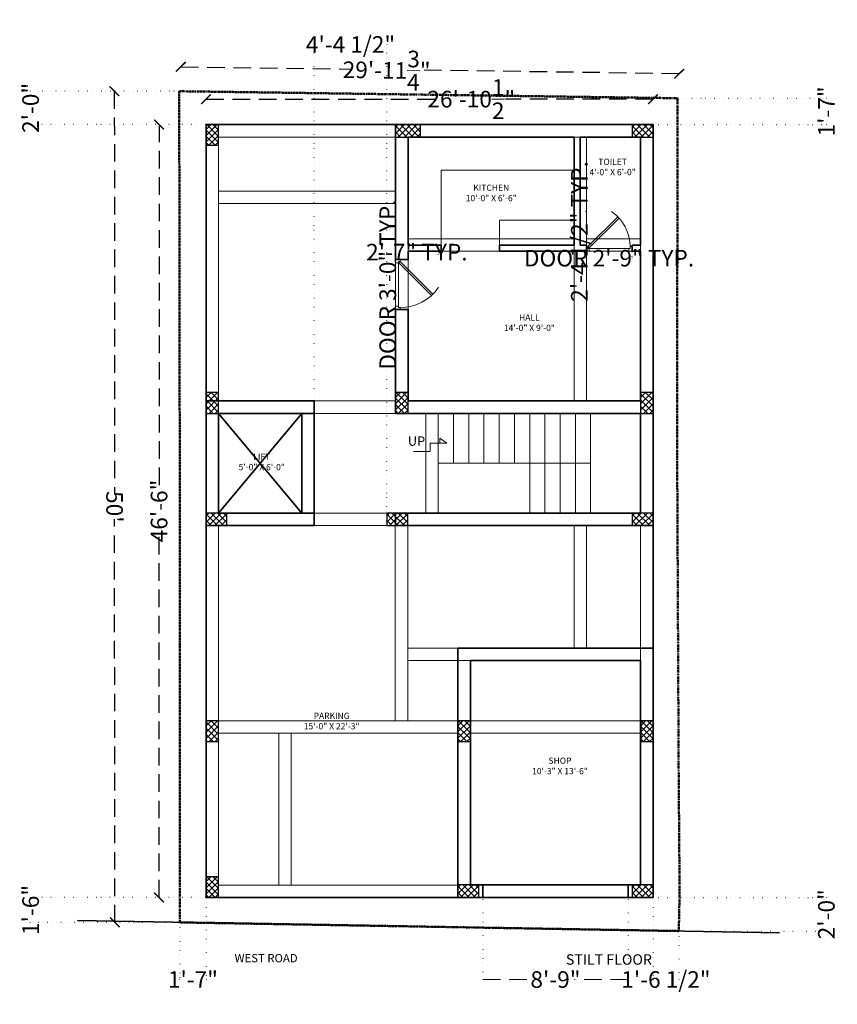
# Model space of a CAD drawing. Units: inches. Extents: x -16911 to -9621, y -48626 to -46270.
# Tile 10 of 20: x -12796 to -12206, y -47022 to -46311. Entities that reach past the tile are written whole.
import ezdxf

# ---------------------------------------------------------------- set-up
doc = ezdxf.new("R2010")
doc.units = ezdxf.units.IN
for name, pattern in [('DASHDOT', [1, 0.5, -0.25, 0, -0.25]), ('DASHED', [19.05, 12.7, -6.35]), ('DOT2', [3.175, 0, -3.175])]:
    doc.linetypes.add(name, pattern=pattern)
for name, color, linetype, lineweight in [('A-ANNO-DIMS', 2, 'Continuous', 13), ('A-ANNO-SYMB', 3, 'Continuous', 13), ('A-ANNO-TEXT', 7, 'Continuous', 18), ('A-AREA-IDEN', 3, 'Continuous', 18), ('A-DOOR', 4, 'Continuous', 18), ('A-FLOR-STRS', 3, 'Continuous', 18), ('A-FURN', 8, 'Continuous', 13), ('A-WALL', 7, 'Continuous', 35), ('C-PROP', 6, 'DASHDOT', 50), ('column', 12, 'Continuous', 30), ('DOOR', 143, 'Continuous', 9), ('EXT BEAM', 132, 'Continuous', 13), ('S-BEAM', 132, 'Continuous', 25), ('S-COLS', 1, 'Continuous', 30), ('STAIRCASE', 137, 'Continuous', 5)]:
    doc.layers.add(name, color=color, linetype=linetype, lineweight=lineweight)
doc.styles.get("Standard").update_dxf_attribs({"font": 'swissel.ttf'})
doc.styles.add('style9', font='swisscl.ttf', dxfattribs={"height": 12})
doc.dimstyles.new('Dim9', dxfattribs={"dimtxt": 10, "dimasz": 0.199219, "dimexe": 1, "dimexo": 0.5, "dimgap": 1, "dimtad": 0, "dimdec": 1, "dimzin": 0, "dimdsep": 46, "dimlunit": 4, "dimtxsty": 'style9', "dimblk": 'ARCHTICK', "dimcen": 0.09, "dimclrd": 256, "dimclrt": 256, "dimadec": 0, "dimazin": 0, "dimtfac": 1, "dimtdec": 1, "dimtix": 1, "dimtofl": 0, "dimtmove": 1, "dimatfit": 3, "dimfxl": 9, "dimtolj": 1, "dimtzin": 0, "dimlwd": -1, "dimarcsym": 0})

# ---------------------------------------------------------------- blocks, each defined once
blk = doc.blocks.new('_ArchTick')
at = {"color": 0, "linetype": 'ByBlock', "const_width": 0.15}
blk.add_lwpolyline([(-0.5, -0.5), (0.5, 0.5)], dxfattribs=at)
blk = doc.blocks.new('*D9')
at = {"layer": 'A-ANNO-DIMS', "color": 0, "linetype": 'DOT2', "lineweight": -2, "transparency": 16777216}
for p, q in [((-12679.71, -46345.34), (-12679.69, -46344.15)), ((-12320.05, -46350.39), (-12320.03, -46349.2))]:
    blk.add_line(p, q, dxfattribs=at)
at = {"layer": 'A-ANNO-DIMS', "color": 0, "linetype": 'DASHED', "lineweight": 25, "transparency": 16777216}
for p, q in [((-12679.71, -46345.15), (-12555.97, -46346.89)), ((-12320.04, -46350.2), (-12506.38, -46347.59))]:
    blk.add_line(p, q, dxfattribs=at)
at = {"layer": 'Defpoints', "color": 0, "transparency": 16777216}
for p in [(-12320.04, -46350.2), (-12679.9, -46359.07), (-12320.24, -46364.11)]:
    blk.add_point(p, dxfattribs=at)
at = {"layer": 'A-ANNO-DIMS', "color": 0, "lineweight": 25, "transparency": 16777216, "xscale": 7, "yscale": 7, "zscale": 7}
for p, rotation in [((-12679.71, -46345.15), 179.1963905603631), ((-12320.04, -46350.2), 359.196390560363)]:
    blk.add_blockref('_ArchTick', p, dxfattribs=dict(at, rotation=rotation))
at = {"layer": 'A-ANNO-DIMS', "color": 0, "transparency": 16777216, "insert": (-12531.18, -46347.68), "char_height": 12, "attachment_point": 5, "rotation": 359.19639, "style": 'style9'}
blk.add_mtext('\\A1;29\'-11{\\H1x;\\S3/4;}"', dxfattribs=at)
blk = doc.blocks.new('*D10')
at = {"layer": 'A-ANNO-DIMS', "color": 0, "linetype": 'DOT2', "lineweight": -2, "transparency": 16777216}
for p, q in [((-12727.5, -46362.82), (-12728.69, -46362.82)), ((-12727.14, -46962.82), (-12728.32, -46962.82))]:
    blk.add_line(p, q, dxfattribs=at)
at = {"layer": 'A-ANNO-DIMS', "color": 0, "linetype": 'DASHED', "lineweight": 25, "transparency": 16777216}
for p, q in [((-12727.69, -46362.82), (-12727.51, -46653.98)), ((-12727.32, -46962.82), (-12727.5, -46671.67))]:
    blk.add_line(p, q, dxfattribs=at)
at = {"layer": 'Defpoints', "color": 0, "transparency": 16777216}
for p in [(-12727.69, -46362.82), (-12708.87, -46362.81), (-12708.51, -46962.81)]:
    blk.add_point(p, dxfattribs=at)
at = {"layer": 'A-ANNO-DIMS', "color": 0, "lineweight": 25, "transparency": 16777216, "xscale": 7, "yscale": 7, "zscale": 7}
for p, rotation in [((-12727.69, -46362.82), 90.0346840750536), ((-12727.32, -46962.82), 270.0346840750536)]:
    blk.add_blockref('_ArchTick', p, dxfattribs=dict(at, rotation=rotation))
at = {"layer": 'A-ANNO-DIMS', "color": 0, "transparency": 16777216, "insert": (-12727.51, -46662.82), "char_height": 12, "attachment_point": 5, "rotation": 270.03468, "style": 'style9'}
blk.add_mtext("\\A1;50'", dxfattribs=at)
blk = doc.blocks.new('*D11')
at = {"layer": 'A-ANNO-DIMS', "color": 0, "linetype": 'DOT2', "lineweight": -2, "transparency": 16777216}
for p, q in [((-12661.47, -46368.33), (-12661.47, -46369.52)), ((-12338.92, -46368.33), (-12338.92, -46369.52))]:
    blk.add_line(p, q, dxfattribs=at)
at = {"layer": 'A-ANNO-DIMS', "color": 0, "linetype": 'DASHED', "lineweight": 25, "transparency": 16777216}
for p, q in [((-12661.47, -46368.52), (-12494.69, -46368.52)), ((-12338.92, -46368.52), (-12445.42, -46368.52))]:
    blk.add_line(p, q, dxfattribs=at)
at = {"layer": 'Defpoints', "color": 0, "transparency": 16777216}
for p in [(-12661.47, -46345.28), (-12338.92, -46345.28), (-12338.92, -46368.52)]:
    blk.add_point(p, dxfattribs=at)
at = {"layer": 'A-ANNO-DIMS', "color": 0, "lineweight": 25, "transparency": 16777216, "xscale": 7, "yscale": 7, "zscale": 7, "rotation": 180}
blk.add_blockref('_ArchTick', (-12661.47, -46368.52), dxfattribs=at)
at = {"layer": 'A-ANNO-DIMS', "color": 0, "lineweight": 25, "transparency": 16777216, "xscale": 7, "yscale": 7, "zscale": 7}
blk.add_blockref('_ArchTick', (-12338.92, -46368.52), dxfattribs=at)
at = {"layer": 'A-ANNO-DIMS', "color": 0, "transparency": 16777216, "insert": (-12470.06, -46368.52), "char_height": 12, "attachment_point": 5, "style": 'style9'}
blk.add_mtext('\\A1;26\'-10{\\H1x;\\S1/2;}"', dxfattribs=at)
blk = doc.blocks.new('*D16')
at = {"layer": 'A-ANNO-DIMS', "color": 0, "linetype": 'DOT2', "lineweight": -2, "transparency": 16777216}
for p, q in [((-12695.22, -46386.86), (-12696.4, -46386.86)), ((-12695.22, -46944.81), (-12696.4, -46944.81))]:
    blk.add_line(p, q, dxfattribs=at)
at = {"layer": 'A-ANNO-DIMS', "color": 0, "linetype": 'DASHED', "lineweight": 25, "transparency": 16777216}
for p, q in [((-12695.4, -46386.86), (-12695.4, -46648.2)), ((-12695.4, -46944.81), (-12695.4, -46683.47))]:
    blk.add_line(p, q, dxfattribs=at)
at = {"layer": 'Defpoints', "color": 0, "transparency": 16777216}
for p in [(-12661.47, -46386.86), (-12695.4, -46944.81), (-12661.47, -46944.81)]:
    blk.add_point(p, dxfattribs=at)
at = {"layer": 'A-ANNO-DIMS', "color": 0, "lineweight": 25, "transparency": 16777216, "xscale": 7, "yscale": 7, "zscale": 7}
for p, rotation in [((-12695.4, -46386.86), 90), ((-12695.4, -46944.81), 270)]:
    blk.add_blockref('_ArchTick', p, dxfattribs=dict(at, rotation=rotation))
at = {"layer": 'A-ANNO-DIMS', "color": 0, "transparency": 16777216, "insert": (-12695.4, -46665.83), "char_height": 12, "attachment_point": 5, "rotation": 90, "style": 'style9'}
blk.add_mtext('\\A1;46\'-6"', dxfattribs=at)
blk = doc.blocks.new('THYHYTJ')
at = {"layer": 'STAIRCASE', "ltscale": 10}
for p, q in [((-7981.18, -46346.18), (-7984.62, -46351.1)), ((-7981.18, -46358.18), (-7981.18, -46346.18)), ((-7984.62, -46351.1), (-7981.18, -46351.1)), ((-7975.18, -46358.18), (-7981.18, -46358.18)), ((-7975.18, -46370.18), (-7975.18, -46358.18))]:
    blk.add_line(p, q, dxfattribs=at)
blk = doc.blocks.new('A$C1C9D3E54')
at = {"layer": 'DOOR'}
blk.add_line((18676.53, 5780.72), (18710.53, 5780.72), dxfattribs=at)
blk.add_lwpolyline([(18685.01, 5806.62), (18710.47, 5781.16), (18711.53, 5782.22), (18686.07, 5807.68), (18685.01, 5806.62)], dxfattribs=at)
blk.add_lwpolyline([(18674.03, 5778.22), (18676.03, 5778.22), (18674.03, 5778.22), (18674.03, 5782.22), (18675.53, 5782.22), (18675.53, 5780.72), (18676.53, 5780.72), (18676.53, 5778.72), (18676.41, 5778.72), (18676.41, 5778.6, -0.414214), (18676.16, 5778.35), (18676.03, 5778.35), (18676.03, 5778.22)], format="xyb", dxfattribs=at)
blk.add_lwpolyline([(18713.03, 5782.22), (18711.53, 5782.22), (18711.53, 5780.72), (18710.53, 5780.72), (18710.53, 5778.72), (18710.66, 5778.72), (18710.66, 5778.6, 0.414214), (18710.91, 5778.35), (18711.03, 5778.35), (18711.03, 5778.22), (18713.03, 5778.22), (18711.03, 5778.22), (18713.03, 5778.22), (18713.03, 5782.22)], format="xyb", close=True, dxfattribs=at)
blk.add_arc((18711.53, 5782.22), 36, 124.03362, 180, dxfattribs=at)
blk = doc.blocks.new('COLUMNS')
at = {"layer": 'column'}
h = blk.add_hatch(dxfattribs=at)
h.set_pattern_fill('ANSI37', color=256, angle=-720)
h.set_pattern_definition([(45, (21703.4588, -104481.6704), (-2.24506403, 2.24506403), []), (135, (21703.4588, -104481.6704), (-2.24506403, -2.24506403), [])])
h.paths.add_polyline_path([(-12061.47, -46401.86), (-12052.47, -46401.86), (-12052.47, -46386.86), (-12061.47, -46386.86)])
h = blk.add_hatch(dxfattribs=at)
h.set_pattern_fill('ANSI37', color=256, angle=-810)
h.set_pattern_definition([(315, (-70004.5392, -80151.7886), (2.24506403, 2.24506403), []), (45, (-70004.5392, -80151.7886), (-2.24506403, 2.24506403), [])])
h.paths.add_polyline_path([(-11924.72, -46386.86), (-11924.72, -46395.86), (-11906.72, -46395.86), (-11906.72, -46386.86)])
h = blk.add_hatch(dxfattribs=at)
h.set_pattern_fill('ANSI37', color=256, angle=-810)
h.set_pattern_definition([(315, (-69833.7395, -80151.7886), (2.24506403, 2.24506403), []), (45, (-69833.7395, -80151.7886), (-2.24506403, 2.24506403), [])])
h.paths.add_polyline_path([(-11753.92, -46386.86), (-11753.92, -46395.86), (-11738.92, -46395.86), (-11738.92, -46386.86)])
h = blk.add_hatch(dxfattribs=at)
h.set_pattern_fill('ANSI37', color=256, angle=-900)
h.set_pattern_definition([(225, (-45817.4075, 11499.4594), (2.24506403, -2.24506403), []), (315, (-45817.4075, 11499.4594), (2.24506403, 2.24506403), [])])
h.paths.add_polyline_path([(-12052.47, -46580.36), (-12061.47, -46580.36), (-12061.47, -46595.36), (-12052.47, -46595.36)])
h = blk.add_hatch(dxfattribs=at)
h.set_pattern_fill('ANSI37', color=256, angle=-720)
h.set_pattern_definition([(45, (21840.2088, -104675.1704), (-2.24506403, 2.24506403), []), (135, (21840.2088, -104675.1704), (-2.24506403, -2.24506403), [])])
h.paths.add_polyline_path([(-11924.72, -46595.36), (-11915.72, -46595.36), (-11915.72, -46580.36), (-11924.72, -46580.36)])
h = blk.add_hatch(dxfattribs=at)
h.set_pattern_fill('ANSI37', color=256, angle=-900)
h.set_pattern_definition([(225, (-45503.8578, 11499.4594), (2.24506403, -2.24506403), []), (315, (-45503.8578, 11499.4594), (2.24506403, 2.24506403), [])])
h.paths.add_polyline_path([(-11738.92, -46580.36), (-11747.92, -46580.36), (-11747.92, -46595.36), (-11738.92, -46595.36)])
h = blk.add_hatch(dxfattribs=at)
h.set_pattern_fill('ANSI37', color=256, angle=-810)
h.set_pattern_definition([(315, (-70141.2892, -80432.2886), (2.24506403, 2.24506403), []), (45, (-70141.2892, -80432.2886), (-2.24506403, 2.24506403), [])])
h.paths.add_polyline_path([(-12061.47, -46667.36), (-12061.47, -46676.36), (-12046.47, -46676.36), (-12046.47, -46667.36)])
h = blk.add_hatch(dxfattribs=at)
h.set_pattern_fill('ANSI37', color=256, angle=-810)
h.set_pattern_definition([(315, (-70010.7892, -80432.2886), (2.24506403, 2.24506403), []), (45, (-70010.7892, -80432.2886), (-2.24506403, 2.24506403), [])])
h.paths.add_polyline_path([(-11930.97, -46667.36), (-11930.97, -46676.36), (-11915.97, -46676.36), (-11915.97, -46667.36)])
h = blk.add_hatch(dxfattribs=at)
h.set_pattern_fill('ANSI37', color=256, angle=-810)
h.set_pattern_definition([(315, (-69833.7395, -80432.2886), (2.24506403, 2.24506403), []), (45, (-69833.7395, -80432.2886), (-2.24506403, 2.24506403), [])])
h.paths.add_polyline_path([(-11753.92, -46667.36), (-11753.92, -46676.36), (-11738.92, -46676.36), (-11738.92, -46667.36)])
h = blk.add_hatch(dxfattribs=at)
h.set_pattern_fill('ANSI37', color=256, angle=-540)
h.set_pattern_definition([(225, (-45817.4075, 11262.5055), (2.24506403, -2.24506403), []), (315, (-45817.4075, 11262.5055), (2.24506403, 2.24506403), [])])
h.paths.add_polyline_path([(-12052.47, -46817.31), (-12061.47, -46817.31), (-12061.47, -46832.31), (-12052.47, -46832.31)])
h = blk.add_hatch(dxfattribs=at)
h.set_pattern_fill('ANSI37', color=256, angle=-720)
h.set_pattern_definition([(45, (21885.2088, -104912.1242), (-2.24506403, 2.24506403), []), (135, (21885.2088, -104912.1242), (-2.24506403, -2.24506403), [])])
h.paths.add_polyline_path([(-11879.72, -46832.31), (-11870.72, -46832.31), (-11870.72, -46817.31), (-11879.72, -46817.31)])
h = blk.add_hatch(dxfattribs=at)
h.set_pattern_fill('ANSI37', color=256, angle=-720)
h.set_pattern_definition([(45, (22017.1023, -104912.1242), (-2.24506403, 2.24506403), []), (135, (22017.1023, -104912.1242), (-2.24506403, -2.24506403), [])])
h.paths.add_polyline_path([(-11747.83, -46832.31), (-11738.83, -46832.31), (-11738.83, -46817.31), (-11747.83, -46817.31)])
h = blk.add_hatch(dxfattribs=at)
h.set_pattern_fill('ANSI37', color=256, angle=-720)
h.set_pattern_definition([(45, (21703.4588, -105024.6242), (-2.24506403, 2.24506403), []), (135, (21703.4588, -105024.6242), (-2.24506403, -2.24506403), [])])
h.paths.add_polyline_path([(-12061.47, -46944.81), (-12052.47, -46944.81), (-12052.47, -46929.81), (-12061.47, -46929.81)])
h = blk.add_hatch(dxfattribs=at)
h.set_pattern_fill('ANSI37', color=256, angle=-810)
h.set_pattern_definition([(315, (-69959.5392, -80700.7425), (2.24506403, 2.24506403), []), (45, (-69959.5392, -80700.7425), (-2.24506403, 2.24506403), [])])
h.paths.add_polyline_path([(-11879.72, -46935.81), (-11879.72, -46944.81), (-11864.72, -46944.81), (-11864.72, -46935.81)])
h = blk.add_hatch(dxfattribs=at)
h.set_pattern_fill('ANSI37', color=256, angle=-810)
h.set_pattern_definition([(315, (-69833.7395, -80700.7425), (2.24506403, 2.24506403), []), (45, (-69833.7395, -80700.7425), (-2.24506403, 2.24506403), [])])
h.paths.add_polyline_path([(-11753.92, -46935.81), (-11753.92, -46944.81), (-11738.92, -46944.81), (-11738.92, -46935.81)])
at = {"layer": 'column', "ltscale": 0.05}
for points in [[(-12052.47, -46386.86), (-12061.47, -46386.86), (-12061.47, -46401.86), (-12052.47, -46401.86)], [(-11906.72, -46395.86), (-11906.72, -46386.86), (-11924.72, -46386.86), (-11924.72, -46395.86)], [(-11738.92, -46395.86), (-11738.92, -46386.86), (-11753.92, -46386.86), (-11753.92, -46395.86)], [(-12061.47, -46595.36), (-12052.47, -46595.36), (-12052.47, -46580.36), (-12061.47, -46580.36)], [(-11915.72, -46580.36), (-11924.72, -46580.36), (-11924.72, -46595.36), (-11915.72, -46595.36)], [(-11747.92, -46595.36), (-11738.92, -46595.36), (-11738.92, -46580.36), (-11747.92, -46580.36)], [(-12046.47, -46676.36), (-12046.47, -46667.36), (-12061.47, -46667.36), (-12061.47, -46676.36)], [(-11915.97, -46676.36), (-11915.97, -46667.36), (-11930.97, -46667.36), (-11930.97, -46676.36)], [(-11738.92, -46676.36), (-11738.92, -46667.36), (-11753.92, -46667.36), (-11753.92, -46676.36)], [(-12061.47, -46832.31), (-12052.47, -46832.31), (-12052.47, -46817.31), (-12061.47, -46817.31)], [(-11870.72, -46817.31), (-11879.72, -46817.31), (-11879.72, -46832.31), (-11870.72, -46832.31)], [(-11738.83, -46817.31), (-11747.83, -46817.31), (-11747.83, -46832.31), (-11738.83, -46832.31)], [(-12052.47, -46929.81), (-12061.47, -46929.81), (-12061.47, -46944.81), (-12052.47, -46944.81)], [(-11864.72, -46944.81), (-11864.72, -46935.81), (-11879.72, -46935.81), (-11879.72, -46944.81)], [(-11738.92, -46944.81), (-11738.92, -46935.81), (-11753.92, -46935.81), (-11753.92, -46944.81)]]:
    blk.add_lwpolyline(points, close=True, dxfattribs=at)
blk = doc.blocks.new('TYPICAL BEAMS G-2')
at = {"layer": 'EXT BEAM'}
for p, q in [((-12061.47, -47658.74), (-11738.92, -47658.74)), ((-12061.47, -48216.7), (-12061.47, -47658.74)), ((-11738.92, -48216.7), (-11738.92, -47658.74)), ((-12052.47, -47667.74), (-11924.72, -47667.74)), ((-12052.47, -47939.24), (-12052.47, -47667.74)), ((-11924.72, -47667.74), (-11924.72, -47858.24)), ((-11915.72, -47667.74), (-11747.92, -47667.74)), ((-11915.72, -47667.74), (-11915.72, -47858.24)), ((-11795.92, -47667.74), (-11795.92, -47858.24)), ((-11786.92, -47667.74), (-11786.92, -47858.24)), ((-11747.92, -47858.24), (-11747.92, -47667.74)), ((-12052.47, -47706.74), (-11924.72, -47706.74)), ((-12052.47, -47715.74), (-11924.72, -47715.74)), ((-11915.72, -47741.24), (-11795.92, -47741.24)), ((-11786.92, -47741.24), (-11747.92, -47741.24)), ((-11915.72, -47750.24), (-11795.92, -47750.24)), ((-11786.92, -47750.24), (-11747.92, -47750.24)), ((-12052.47, -47858.24), (-11924.72, -47858.24)), ((-11915.72, -47858.24), (-11747.92, -47858.24)), ((-12052.47, -47867.24), (-11924.72, -47867.24)), ((-11992.47, -47867.24), (-11992.47, -47939.24)), ((-11983.47, -47867.24), (-11983.47, -47939.24)), ((-11915.72, -47867.24), (-11747.92, -47867.24)), ((-11902.92, -47867.24), (-11902.92, -47939.24)), ((-11893.92, -47867.24), (-11893.92, -47939.24)), ((-11747.92, -47939.24), (-11747.92, -47867.24)), ((-12046.47, -47939.24), (-11929.47, -47939.24)), ((-11920.47, -47939.24), (-11738.92, -47939.24)), ((-12052.47, -48089.2), (-12052.47, -47948.24)), ((-12046.47, -47948.24), (-11929.47, -47948.24)), ((-11924.97, -47948.24), (-11924.97, -48089.2)), ((-11920.47, -47948.24), (-11738.92, -47948.24)), ((-11915.97, -47948.24), (-11915.97, -48089.2)), ((-11795.92, -47948.24), (-11795.92, -48036.7)), ((-11786.92, -47948.24), (-11786.92, -48036.7)), ((-11747.92, -48089.2), (-11747.92, -47948.24)), ((-11747.92, -48036.7), (-11915.97, -48036.7)), ((-11747.92, -48045.7), (-11915.97, -48045.7)), ((-12052.47, -48089.2), (-11747.92, -48089.2)), ((-12052.47, -48216.7), (-12052.47, -48098.2)), ((-12052.47, -48098.2), (-11879.72, -48098.2)), ((-12008.97, -48098.2), (-12008.97, -48207.7)), ((-11999.97, -48098.2), (-11999.97, -48207.7)), ((-11879.72, -48098.2), (-11879.72, -48207.7)), ((-11870.72, -48098.2), (-11747.92, -48098.2)), ((-11870.72, -48098.2), (-11870.72, -48207.7)), ((-11747.92, -48207.7), (-11747.92, -48098.2)), ((-12052.47, -48207.7), (-11879.72, -48207.7)), ((-11870.72, -48207.7), (-11747.92, -48207.7)), ((-12061.47, -48216.7), (-11738.92, -48216.7))]:
    blk.add_line(p, q, dxfattribs=at)
blk = doc.blocks.new('*D65')
at = {"layer": 'A-ANNO-DIMS', "color": 0, "linetype": 'DOT2', "lineweight": -2, "transparency": 16777216}
for p, q in [((-12525.47, -46484.36), (-12531.37, -46484.36)), ((-12525.47, -46520.36), (-12531.37, -46520.36))]:
    blk.add_line(p, q, dxfattribs=at)
at = {"layer": 'A-ANNO-DIMS', "linetype": 'DASHED', "transparency": 16777216}
for p, q in [((-12530.37, -46484.36), (-12530.37, -46484.16)), ((-12530.37, -46520.36), (-12530.37, -46520.55))]:
    blk.add_line(p, q, dxfattribs=at)
at = {"layer": 'Defpoints', "color": 0, "transparency": 16777216}
for p in [(-12530.37, -46484.36), (-12524.97, -46484.36), (-12524.97, -46520.36)]:
    blk.add_point(p, dxfattribs=at)
at = {"layer": 'A-ANNO-DIMS', "transparency": 16777216, "xscale": 0.19921875, "yscale": 0.19921875, "zscale": 0.19921875}
for p, rotation in [((-12530.37, -46484.36), 270), ((-12530.37, -46520.36), 90)]:
    blk.add_blockref('_ArchTick', p, dxfattribs=dict(at, rotation=rotation))
at = {"layer": 'A-ANNO-DIMS', "transparency": 16777216, "insert": (-12530.37, -46502.36), "char_height": 12, "attachment_point": 5, "rotation": 90, "style": 'style9'}
blk.add_mtext('\\A1;DOOR 3\'-0" TYP.', dxfattribs=at)
blk = doc.blocks.new('*D66')
at = {"layer": 'A-ANNO-DIMS', "linetype": 'DASHED', "transparency": 16777216}
for p, q in [((-12524.97, -46478.96), (-12525.17, -46478.96)), ((-12493.75, -46478.96), (-12493.55, -46478.96))]:
    blk.add_line(p, q, dxfattribs=at)
at = {"layer": 'A-ANNO-DIMS', "color": 0, "linetype": 'DOT2', "lineweight": -2, "transparency": 16777216}
for p, q in [((-12524.97, -46483.86), (-12524.97, -46477.96)), ((-12493.75, -46483.86), (-12493.75, -46477.96))]:
    blk.add_line(p, q, dxfattribs=at)
at = {"layer": 'Defpoints', "color": 0, "transparency": 16777216}
for p in [(-12524.97, -46484.36), (-12493.75, -46478.96), (-12493.75, -46484.36)]:
    blk.add_point(p, dxfattribs=at)
at = {"layer": 'A-ANNO-DIMS', "transparency": 16777216, "xscale": 0.19921875, "yscale": 0.19921875, "zscale": 0.19921875}
blk.add_blockref('_ArchTick', (-12524.97, -46478.96), dxfattribs=at)
at = {"layer": 'A-ANNO-DIMS', "transparency": 16777216, "xscale": 0.19921875, "yscale": 0.19921875, "zscale": 0.19921875, "rotation": 180}
blk.add_blockref('_ArchTick', (-12493.75, -46478.96), dxfattribs=at)
at = {"layer": 'A-ANNO-DIMS', "transparency": 16777216, "insert": (-12509.36, -46478.96), "char_height": 12, "attachment_point": 5, "style": 'style9'}
blk.add_mtext('\\A1;2\'-7" TYP.', dxfattribs=at)
blk = doc.blocks.new('*D67')
at = {"layer": 'A-ANNO-DIMS', "linetype": 'DASHED', "transparency": 16777216}
for p, q in [((-12387.17, -46483.31), (-12387.37, -46483.31)), ((-12354.17, -46483.31), (-12353.98, -46483.31))]:
    blk.add_line(p, q, dxfattribs=at)
at = {"layer": 'A-ANNO-DIMS', "color": 0, "linetype": 'DOT2', "lineweight": -2, "transparency": 16777216}
for p, q in [((-12387.17, -46478.86), (-12387.17, -46484.31)), ((-12354.17, -46478.86), (-12354.17, -46484.31))]:
    blk.add_line(p, q, dxfattribs=at)
at = {"layer": 'Defpoints', "color": 0, "transparency": 16777216}
for p in [(-12387.17, -46478.36), (-12387.17, -46483.31), (-12354.17, -46478.36)]:
    blk.add_point(p, dxfattribs=at)
at = {"layer": 'A-ANNO-DIMS', "transparency": 16777216, "xscale": 0.19921875, "yscale": 0.19921875, "zscale": 0.19921875}
blk.add_blockref('_ArchTick', (-12387.17, -46483.31), dxfattribs=at)
at = {"layer": 'A-ANNO-DIMS', "transparency": 16777216, "xscale": 0.19921875, "yscale": 0.19921875, "zscale": 0.19921875, "rotation": 180}
blk.add_blockref('_ArchTick', (-12354.17, -46483.31), dxfattribs=at)
at = {"layer": 'A-ANNO-DIMS', "transparency": 16777216, "insert": (-12370.67, -46483.31), "char_height": 12, "attachment_point": 5, "style": 'style9'}
blk.add_mtext('\\A1;DOOR 2\'-9" TYP.', dxfattribs=at)
blk = doc.blocks.new('*D68')
at = {"layer": 'A-ANNO-DIMS', "color": 0, "linetype": 'DOT2', "lineweight": -2, "transparency": 16777216}
for p, q in [((-12387.67, -46449.73), (-12393.12, -46449.73)), ((-12387.67, -46478.36), (-12393.12, -46478.36))]:
    blk.add_line(p, q, dxfattribs=at)
at = {"layer": 'A-ANNO-DIMS', "linetype": 'DASHED', "transparency": 16777216}
for p, q in [((-12392.12, -46449.73), (-12392.12, -46449.53)), ((-12392.12, -46478.36), (-12392.12, -46478.55))]:
    blk.add_line(p, q, dxfattribs=at)
at = {"layer": 'Defpoints', "color": 0, "transparency": 16777216}
for p in [(-12392.12, -46449.73), (-12387.17, -46449.73), (-12387.17, -46478.36)]:
    blk.add_point(p, dxfattribs=at)
at = {"layer": 'A-ANNO-DIMS', "transparency": 16777216, "xscale": 0.19921875, "yscale": 0.19921875, "zscale": 0.19921875}
for p, rotation in [((-12392.12, -46449.73), 270), ((-12392.12, -46478.36), 90)]:
    blk.add_blockref('_ArchTick', p, dxfattribs=dict(at, rotation=rotation))
at = {"layer": 'A-ANNO-DIMS', "transparency": 16777216, "insert": (-12392.12, -46464.04), "char_height": 12, "attachment_point": 5, "rotation": 90, "style": 'style9'}
blk.add_mtext('\\A1;2\'-4 1/2" TYP.', dxfattribs=at)
blk = doc.blocks.new('*D106')
at = {"layer": 'A-ANNO-DIMS', "color": 0, "linetype": 'DOT2', "lineweight": -2, "transparency": 16777216}
for p, q in [((-12681.34, -46362.81), (-12789.1, -46362.81)), ((-12661.97, -46386.86), (-12789.1, -46386.86))]:
    blk.add_line(p, q, dxfattribs=at)
at = {"layer": 'A-ANNO-DIMS', "linetype": 'DASHED', "transparency": 16777216}
for p, q in [((-12788.1, -46362.81), (-12788.1, -46362.61)), ((-12788.1, -46386.86), (-12788.1, -46387.05))]:
    blk.add_line(p, q, dxfattribs=at)
at = {"layer": 'Defpoints', "color": 0, "transparency": 16777216}
for p in [(-12680.84, -46362.81), (-12788.1, -46386.86), (-12661.47, -46386.86)]:
    blk.add_point(p, dxfattribs=at)
at = {"layer": 'A-ANNO-DIMS', "transparency": 16777216, "xscale": 0.19921875, "yscale": 0.19921875, "zscale": 0.19921875}
for p, rotation in [((-12788.1, -46362.81), 270), ((-12788.1, -46386.86), 90)]:
    blk.add_blockref('_ArchTick', p, dxfattribs=dict(at, rotation=rotation))
at = {"layer": 'A-ANNO-DIMS', "transparency": 16777216, "insert": (-12788.1, -46374.83), "char_height": 12, "attachment_point": 5, "rotation": 90, "style": 'style9'}
blk.add_mtext('\\A1;2\'-0"', dxfattribs=at)
blk = doc.blocks.new('*D107')
at = {"layer": 'A-ANNO-DIMS', "color": 0, "linetype": 'DOT2', "lineweight": -2, "transparency": 16777216}
for p, q in [((-12320.67, -46367.86), (-12212.8, -46367.86)), ((-12338.42, -46386.86), (-12212.8, -46386.86))]:
    blk.add_line(p, q, dxfattribs=at)
at = {"layer": 'A-ANNO-DIMS', "linetype": 'DASHED', "transparency": 16777216}
for p, q in [((-12213.8, -46367.86), (-12213.8, -46367.66)), ((-12213.8, -46386.86), (-12213.8, -46387.05))]:
    blk.add_line(p, q, dxfattribs=at)
at = {"layer": 'Defpoints', "color": 0, "transparency": 16777216}
for p in [(-12321.17, -46367.86), (-12338.92, -46386.86), (-12213.8, -46386.86)]:
    blk.add_point(p, dxfattribs=at)
at = {"layer": 'A-ANNO-DIMS', "transparency": 16777216, "xscale": 0.19921875, "yscale": 0.19921875, "zscale": 0.19921875}
for p, rotation in [((-12213.8, -46367.86), 270), ((-12213.8, -46386.86), 90)]:
    blk.add_blockref('_ArchTick', p, dxfattribs=dict(at, rotation=rotation))
at = {"layer": 'A-ANNO-DIMS', "transparency": 16777216, "insert": (-12213.8, -46377.36), "char_height": 12, "attachment_point": 5, "rotation": 90, "style": 'style9'}
blk.add_mtext('\\A1;1\'-7"', dxfattribs=at)
blk = doc.blocks.new('*D108')
at = {"layer": 'A-ANNO-DIMS', "color": 0, "linetype": 'DOT2', "lineweight": -2, "transparency": 16777216}
for p, q in [((-12661.97, -46944.81), (-12789.1, -46944.81)), ((-12680.97, -46962.81), (-12789.1, -46962.81))]:
    blk.add_line(p, q, dxfattribs=at)
at = {"layer": 'A-ANNO-DIMS', "linetype": 'DASHED', "transparency": 16777216}
for p, q in [((-12788.1, -46944.81), (-12788.1, -46944.61)), ((-12788.1, -46962.81), (-12788.1, -46963.01))]:
    blk.add_line(p, q, dxfattribs=at)
at = {"layer": 'Defpoints', "color": 0, "transparency": 16777216}
for p in [(-12788.1, -46944.81), (-12661.47, -46944.81), (-12680.47, -46962.81)]:
    blk.add_point(p, dxfattribs=at)
at = {"layer": 'A-ANNO-DIMS', "transparency": 16777216, "xscale": 0.19921875, "yscale": 0.19921875, "zscale": 0.19921875}
for p, rotation in [((-12788.1, -46944.81), 270), ((-12788.1, -46962.81), 90)]:
    blk.add_blockref('_ArchTick', p, dxfattribs=dict(at, rotation=rotation))
at = {"layer": 'A-ANNO-DIMS', "transparency": 16777216, "insert": (-12788.1, -46953.81), "char_height": 12, "attachment_point": 5, "rotation": 90, "style": 'style9'}
blk.add_mtext('\\A1;1\'-6"', dxfattribs=at)
blk = doc.blocks.new('*D109')
at = {"layer": 'A-ANNO-DIMS', "color": 0, "linetype": 'DOT2', "lineweight": -2, "transparency": 16777216}
for p, q in [((-12338.42, -46944.81), (-12212.8, -46944.81)), ((-12319.79, -46969.03), (-12212.8, -46969.03))]:
    blk.add_line(p, q, dxfattribs=at)
at = {"layer": 'A-ANNO-DIMS', "linetype": 'DASHED', "transparency": 16777216}
for p, q in [((-12213.8, -46944.81), (-12213.8, -46944.61)), ((-12213.8, -46969.03), (-12213.8, -46969.23))]:
    blk.add_line(p, q, dxfattribs=at)
at = {"layer": 'Defpoints', "color": 0, "transparency": 16777216}
for p in [(-12338.92, -46944.81), (-12213.8, -46944.81), (-12320.29, -46969.03)]:
    blk.add_point(p, dxfattribs=at)
at = {"layer": 'A-ANNO-DIMS', "transparency": 16777216, "xscale": 0.19921875, "yscale": 0.19921875, "zscale": 0.19921875}
for p, rotation in [((-12213.8, -46944.81), 270), ((-12213.8, -46969.03), 90)]:
    blk.add_blockref('_ArchTick', p, dxfattribs=dict(at, rotation=rotation))
at = {"layer": 'A-ANNO-DIMS', "transparency": 16777216, "insert": (-12213.8, -46956.92), "char_height": 12, "attachment_point": 5, "rotation": 90, "style": 'style9'}
blk.add_mtext('\\A1;2\'-0"', dxfattribs=at)
blk = doc.blocks.new('*D110')
at = {"layer": 'A-ANNO-DIMS', "color": 0, "linetype": 'DOT2', "lineweight": -2, "transparency": 16777216}
for p, q in [((-12661.47, -46945.31), (-12661.47, -47005.04)), ((-12680.47, -46963.31), (-12680.47, -47005.04))]:
    blk.add_line(p, q, dxfattribs=at)
at = {"layer": 'A-ANNO-DIMS', "linetype": 'DASHED', "transparency": 16777216}
for p, q in [((-12680.47, -47004.04), (-12680.67, -47004.04)), ((-12661.47, -47004.04), (-12661.28, -47004.04))]:
    blk.add_line(p, q, dxfattribs=at)
at = {"layer": 'Defpoints', "color": 0, "transparency": 16777216}
for p in [(-12661.47, -46944.81), (-12680.47, -46962.81), (-12661.47, -47004.04)]:
    blk.add_point(p, dxfattribs=at)
at = {"layer": 'A-ANNO-DIMS', "transparency": 16777216, "xscale": 0.19921875, "yscale": 0.19921875, "zscale": 0.19921875}
blk.add_blockref('_ArchTick', (-12680.47, -47004.04), dxfattribs=at)
at = {"layer": 'A-ANNO-DIMS', "transparency": 16777216, "xscale": 0.19921875, "yscale": 0.19921875, "zscale": 0.19921875, "rotation": 180}
blk.add_blockref('_ArchTick', (-12661.47, -47004.04), dxfattribs=at)
at = {"layer": 'A-ANNO-DIMS', "transparency": 16777216, "insert": (-12670.97, -47004.04), "char_height": 12, "attachment_point": 5, "style": 'style9'}
blk.add_mtext('\\A1;1\'-7"', dxfattribs=at)
blk = doc.blocks.new('*D111')
at = {"layer": 'A-ANNO-DIMS', "color": 0, "linetype": 'DOT2', "lineweight": -2, "transparency": 16777216}
for p, q in [((-12338.92, -46945.31), (-12338.92, -47005.04)), ((-12320.29, -46969.53), (-12320.29, -47005.04))]:
    blk.add_line(p, q, dxfattribs=at)
at = {"layer": 'A-ANNO-DIMS', "linetype": 'DASHED', "transparency": 16777216}
for p, q in [((-12338.92, -47004.04), (-12339.12, -47004.04)), ((-12320.29, -47004.04), (-12320.09, -47004.04))]:
    blk.add_line(p, q, dxfattribs=at)
at = {"layer": 'Defpoints', "color": 0, "transparency": 16777216}
for p in [(-12338.92, -46944.81), (-12320.29, -46969.03), (-12338.92, -47004.04)]:
    blk.add_point(p, dxfattribs=at)
at = {"layer": 'A-ANNO-DIMS', "transparency": 16777216, "xscale": 0.19921875, "yscale": 0.19921875, "zscale": 0.19921875}
blk.add_blockref('_ArchTick', (-12338.92, -47004.04), dxfattribs=at)
at = {"layer": 'A-ANNO-DIMS', "transparency": 16777216, "xscale": 0.19921875, "yscale": 0.19921875, "zscale": 0.19921875, "rotation": 180}
blk.add_blockref('_ArchTick', (-12320.29, -47004.04), dxfattribs=at)
at = {"layer": 'A-ANNO-DIMS', "transparency": 16777216, "insert": (-12329.61, -47004.04), "char_height": 12, "attachment_point": 5, "style": 'style9'}
blk.add_mtext('\\A1;1\'-6 1/2"', dxfattribs=at)
blk = doc.blocks.new('*D112')
at = {"layer": 'A-ANNO-DIMS', "color": 0, "linetype": 'DOT2', "lineweight": -2, "transparency": 16777216}
for p, q in [((-12461.72, -46936.31), (-12461.72, -47005.04)), ((-12356.92, -46936.31), (-12356.92, -47005.04))]:
    blk.add_line(p, q, dxfattribs=at)
at = {"layer": 'A-ANNO-DIMS', "linetype": 'DASHED', "transparency": 16777216}
for p, q in [((-12461.72, -47004.04), (-12423.14, -47004.04)), ((-12356.92, -47004.04), (-12395.51, -47004.04))]:
    blk.add_line(p, q, dxfattribs=at)
at = {"layer": 'Defpoints', "color": 0, "transparency": 16777216}
for p in [(-12461.72, -46935.81), (-12356.92, -46935.81), (-12356.92, -47004.04)]:
    blk.add_point(p, dxfattribs=at)
at = {"layer": 'A-ANNO-DIMS', "transparency": 16777216, "xscale": 0.19921875, "yscale": 0.19921875, "zscale": 0.19921875, "rotation": 180}
blk.add_blockref('_ArchTick', (-12461.72, -47004.04), dxfattribs=at)
at = {"layer": 'A-ANNO-DIMS', "transparency": 16777216, "xscale": 0.19921875, "yscale": 0.19921875, "zscale": 0.19921875}
blk.add_blockref('_ArchTick', (-12356.92, -47004.04), dxfattribs=at)
at = {"layer": 'A-ANNO-DIMS', "transparency": 16777216, "insert": (-12409.32, -47004.04), "char_height": 12, "attachment_point": 5, "style": 'style9'}
blk.add_mtext('\\A1;8\'-9"', dxfattribs=at)
blk = doc.blocks.new('*D113')
at = {"layer": 'A-ANNO-DIMS', "linetype": 'DASHED', "transparency": 16777216}
for p, q in [((-12583.47, -46329.06), (-12583.67, -46329.06)), ((-12530.97, -46329.06), (-12530.78, -46329.06))]:
    blk.add_line(p, q, dxfattribs=at)
at = {"layer": 'A-ANNO-DIMS', "color": 0, "linetype": 'DOT2', "lineweight": -2, "transparency": 16777216}
for p, q in [((-12583.47, -46675.86), (-12583.47, -46328.06)), ((-12530.97, -46675.86), (-12530.97, -46328.06))]:
    blk.add_line(p, q, dxfattribs=at)
at = {"layer": 'Defpoints', "color": 0, "transparency": 16777216}
for p in [(-12530.97, -46329.06), (-12583.47, -46676.36), (-12530.97, -46676.36)]:
    blk.add_point(p, dxfattribs=at)
at = {"layer": 'A-ANNO-DIMS', "transparency": 16777216, "xscale": 0.19921875, "yscale": 0.19921875, "zscale": 0.19921875}
blk.add_blockref('_ArchTick', (-12583.47, -46329.06), dxfattribs=at)
at = {"layer": 'A-ANNO-DIMS', "transparency": 16777216, "xscale": 0.19921875, "yscale": 0.19921875, "zscale": 0.19921875, "rotation": 180}
blk.add_blockref('_ArchTick', (-12530.97, -46329.06), dxfattribs=at)
at = {"layer": 'A-ANNO-DIMS', "transparency": 16777216, "insert": (-12557.22, -46329.06), "char_height": 12, "attachment_point": 5, "style": 'style9'}
blk.add_mtext('\\A1;4\'-4 1/2"', dxfattribs=at)

msp = doc.modelspace()

# ---------------------------------------------------------------- linework, layer by layer
at = {"layer": 'A-FLOR-STRS', "ltscale": 10}
for p, q in [((-12493.925, -46595.355), (-12493.925, -46631.355)), ((-12482.925, -46595.355), (-12482.925, -46631.355)), ((-12471.925, -46595.355), (-12471.925, -46631.355)), ((-12460.925, -46595.355), (-12460.925, -46631.355)), ((-12449.925, -46595.355), (-12449.925, -46631.355)), ((-12438.925, -46595.355), (-12438.925, -46631.355)), ((-12427.925, -46595.355), (-12427.925, -46667.355)), ((-12416.925, -46595.355), (-12416.925, -46667.355)), ((-12405.925, -46595.355), (-12405.925, -46667.355)), ((-12394.925, -46595.355), (-12394.925, -46667.355)), ((-12383.925, -46595.355), (-12383.925, -46667.355)), ((-12383.925, -46631.355), (-12493.925, -46631.355))]:
    msp.add_line(p, q, dxfattribs=at)
at = {"layer": 'A-FURN', "ltscale": 0.2}
for p, q in [((-12491.724, -46473.855), (-12491.724, -46419.855)), ((-12395.925, -46419.855), (-12491.724, -46419.855)), ((-12449.724, -46473.855), (-12449.724, -46455.855)), ((-12395.925, -46455.855), (-12449.724, -46455.855))]:
    msp.add_line(p, q, dxfattribs=at)
at = {"layer": 'A-WALL'}
for p, q in [((-12661.474, -46586.355), (-12661.474, -46386.855)), ((-12524.724, -46386.855), (-12661.474, -46386.855)), ((-12524.724, -46484.355), (-12524.724, -46386.855)), ((-12524.724, -46386.855), (-12338.925, -46386.855)), ((-12338.925, -46386.855), (-12338.925, -46676.355)), ((-12515.724, -46473.855), (-12515.724, -46395.855)), ((-12395.925, -46395.855), (-12515.724, -46395.855)), ((-12395.925, -46395.855), (-12395.925, -46473.855)), ((-12347.925, -46395.855), (-12391.425, -46395.855)), ((-12391.425, -46395.855), (-12391.425, -46473.855)), ((-12347.925, -46395.855), (-12347.925, -46473.855)), ((-12491.724, -46473.855), (-12515.724, -46473.855)), ((-12491.724, -46478.355), (-12491.724, -46473.855)), ((-12449.724, -46478.355), (-12449.724, -46473.855)), ((-12395.925, -46473.855), (-12449.724, -46473.855)), ((-12386.925, -46473.855), (-12391.425, -46473.855)), ((-12386.925, -46478.355), (-12386.925, -46473.855)), ((-12347.925, -46473.855), (-12353.925, -46473.855)), ((-12353.925, -46478.355), (-12353.925, -46473.855)), ((-12524.724, -46484.355), (-12515.724, -46484.355)), ((-12515.724, -46484.355), (-12515.724, -46478.355)), ((-12491.724, -46478.355), (-12515.724, -46478.355)), ((-12386.925, -46478.355), (-12449.724, -46478.355)), ((-12347.925, -46478.355), (-12353.925, -46478.355)), ((-12347.925, -46478.355), (-12347.925, -46586.355)), ((-12524.724, -46520.355), (-12515.724, -46520.355)), ((-12524.724, -46595.355), (-12524.724, -46520.355)), ((-12515.724, -46586.355), (-12515.724, -46520.355)), ((-12661.474, -46676.355), (-12661.474, -46586.355)), ((-12583.474, -46586.355), (-12661.474, -46586.355)), ((-12583.474, -46595.355), (-12583.474, -46586.355)), ((-12347.925, -46586.355), (-12515.724, -46586.355)), ((-12652.474, -46667.355), (-12652.474, -46595.355)), ((-12583.474, -46595.355), (-12652.474, -46595.355)), ((-12652.474, -46595.355), (-12592.474, -46667.355)), ((-12652.474, -46667.355), (-12592.474, -46595.355)), ((-12592.474, -46667.355), (-12592.474, -46595.355)), ((-12583.474, -46667.355), (-12583.474, -46595.355)), ((-12347.925, -46595.355), (-12524.724, -46595.355)), ((-12347.925, -46595.355), (-12347.925, -46667.355)), ((-12583.474, -46667.355), (-12652.474, -46667.355)), ((-12583.474, -46676.355), (-12583.474, -46667.355)), ((-12347.925, -46667.355), (-12524.724, -46667.355)), ((-12524.724, -46667.355), (-12524.724, -46676.355)), ((-12661.474, -46944.809), (-12661.474, -46676.355)), ((-12583.474, -46676.355), (-12661.474, -46676.355)), ((-12524.974, -46676.355), (-12524.974, -46676.355)), ((-12338.925, -46676.355), (-12524.724, -46676.355)), ((-12338.925, -46676.355), (-12338.925, -46764.809)), ((-12479.724, -46944.809), (-12479.724, -46764.809)), ((-12479.724, -46764.809), (-12338.925, -46764.809)), ((-12338.925, -46764.809), (-12338.925, -46944.809)), ((-12470.724, -46935.809), (-12470.724, -46773.809)), ((-12470.724, -46773.809), (-12347.925, -46773.809)), ((-12347.925, -46773.809), (-12347.925, -46935.809)), ((-12470.724, -46935.809), (-12461.724, -46935.809)), ((-12461.724, -46944.809), (-12461.724, -46935.809)), ((-12461.724, -46935.809), (-12356.925, -46935.809)), ((-12356.925, -46935.809), (-12356.925, -46944.809)), ((-12356.925, -46935.809), (-12347.925, -46935.809)), ((-12661.474, -46944.809), (-12479.724, -46944.809)), ((-12479.724, -46944.809), (-12461.724, -46944.809)), ((-12461.724, -46944.809), (-12356.925, -46944.809)), ((-12356.925, -46944.809), (-12338.925, -46944.809)), ((-12247.547, -46970.292), (-12754.349, -46961.533))]:
    msp.add_line(p, q, dxfattribs=at)
at = {"layer": 'C-PROP'}
msp.add_lwpolyline([(-12680.474, -46962.809), (-12320.293, -46969.035), (-12319.732, -46940.446), (-12320.395, -46855.606), (-12321.561, -46609.511), (-12321.175, -46367.855), (-12680.838, -46362.811), (-12680.3, -46762.955)], close=True, dxfattribs=at)

# ---------------------------------------------------------------- block references
at = {"layer": 'A-ANNO-SYMB', "rotation": 270.0000000000144}
msp.add_blockref('THYHYTJ', (33858.429, -54597.957), dxfattribs=at)
at = {"layer": 'A-DOOR', "xscale": -0.8461538461538624, "yscale": 0.8461538461538624, "zscale": 0.8461538461538624}
msp.add_blockref('A$C1C9D3E54', (3446.928, -51367.622), dxfattribs=at)
at = {"layer": 'A-DOOR', "xscale": -0.9230769230769229, "yscale": 0.9230769230769229, "zscale": 0.9230769230769229, "rotation": 270}
msp.add_blockref('A$C1C9D3E54', (-17858.72, -63757.922), dxfattribs=at)
at = {"layer": 'S-BEAM'}
msp.add_blockref('TYPICAL BEAMS G-2', (-600, 1271.886), dxfattribs=at)
at = {"layer": 'S-COLS'}
msp.add_blockref('COLUMNS', (-600, 0), dxfattribs=at)

# ---------------------------------------------------------------- texts
at = {"layer": 'A-ANNO-TEXT'}
msp.add_text('UP', height=6.75, dxfattribs=at).set_placement((-12515.824, -46618.742))
at = {"layer": 'A-ANNO-TEXT', "ltscale": 10, "attachment_point": 1, "style": 'style9'}
for s, insert, char_height, width in [('\\A1;{\\fCentury Gothic|b0|i0|c0|p34;WEST ROAD}', (-12640.885, -46985.611), 6, 70.69764), ('\\A1;{\\fCentury Gothic|b0|i0|c0|p34;STILT FLOOR}', (-12401.781, -46985.845), 7.5, 166.78033)]:
    msp.add_mtext(s, dxfattribs=dict(at, insert=insert, char_height=char_height, width=width))
at = {"layer": 'A-AREA-IDEN', "ltscale": 10, "char_height": 4.5, "width": 42.823, "attachment_point": 1, "style": 'style9'}
for s, insert in [('\\A1;\\pxqc;{\\fCentury Gothic|b0|i0|c0|p34;TOILET\\P4\'-0" X 6\'-0"}', (-12389.497, -46411.463)), ('\\A1;\\pxqc;{\\fCentury Gothic|b0|i0|c0|p34;KITCHEN\\P10\'-0" X 6\'-6"}', (-12477.09, -46430.204)), ('\\A1;\\pxqc;{\\fCentury Gothic|b0|i0|c0|p34;HALL\\P14\'-0" X 9\'-0"}', (-12449.585, -46523.917)), ('\\A1;\\pxqc;{\\fCentury Gothic|b0|i0|c0|p34;LIFT\\P5\'-0" X 6\'-0"}', (-12642.698, -46624.39)), ('\\A1;\\pxqc;{\\fCentury Gothic|b0|i0|c0|p34;PARKING\\P15\'-0" X 22\'-3"}', (-12592.26, -46811.449)), ('\\A1;\\pxqc;{\\fCentury Gothic|b0|i0|c0|p34;SHOP\\P10\'-3" X 13\'-6"}', (-12427.469, -46843.832))]:
    msp.add_mtext(s, dxfattribs=dict(at, insert=insert))

# ---------------------------------------------------------------- dimensions: what is measured, and where the dimension line sits
at = {"layer": 'A-ANNO-DIMS'}
for base, p1, p2, picture, middle in [((-12530.974, -46329.061), (-12583.474, -46676.355), (-12530.974, -46676.355), '*D113', (-12557.224, -46329.061)), ((-12356.925, -47004.042), (-12461.724, -46935.809), (-12356.925, -46935.809), '*D112', (-12409.324, -47004.042)), ((-12661.474, -47004.042), (-12680.474, -46962.809), (-12661.474, -46944.809), '*D110', (-12670.974, -47004.042)), ((-12338.925, -47004.042), (-12320.293, -46969.035), (-12338.925, -46944.809), '*D111', (-12329.609, -47004.042))]:
    dim = msp.add_linear_dim(base=base, p1=p1, p2=p2, dimstyle='Dim9', override={"dimdec": 1, "dimlfac": 1, "dimrnd": 0, "dimzin": 1, "dimdsep": 46, "dimlunit": 4, "dimfrac": 2}, dxfattribs=at)
    dim.commit()
    dim.dimension.update_dxf_attribs({"geometry": picture, "text_midpoint": middle})
dim = msp.add_linear_dim(base=(-12320.044, -46350.199), p1=(-12679.902, -46359.069), p2=(-12320.239, -46364.114), angle=359.196391, dimstyle='Dim9', override={"dimtxt": 12, "dimasz": 7, "dimdec": 2, "dimclrd": 0, "dimclre": 0, "dimclrt": 0, "dimtdec": 2, "dimfxl": 0.1875, "dimfxlon": 1, "dimlwd": 25, "dimarcsym": 2}, dxfattribs=at)
dim.commit()
dim.dimension.update_dxf_attribs({"geometry": '*D9', "text_midpoint": (-12531.179, -46347.677), "dimtype": 161})
dim = msp.add_linear_dim(base=(-12338.925, -46368.516), p1=(-12661.474, -46345.28), p2=(-12338.925, -46345.28), dimstyle='Dim9', override={"dimtxt": 12, "dimasz": 7, "dimdec": 2, "dimclrd": 0, "dimclre": 0, "dimclrt": 0, "dimtdec": 2, "dimfxl": 0.1875, "dimfxlon": 1, "dimlwd": 25, "dimarcsym": 2}, dxfattribs=at)
dim.commit()
dim.dimension.update_dxf_attribs({"geometry": '*D11', "text_midpoint": (-12470.059, -46368.516), "dimtype": 160})
for base, p1, p2, override, picture, middle in [((-12788.099, -46386.855), (-12680.838, -46362.811), (-12661.474, -46386.855), {"dimdec": 1, "dimlfac": 1, "dimrnd": 0, "dimzin": 1, "dimdsep": 46, "dimlunit": 4, "dimfrac": 2}, '*D106', (-12788.099, -46374.833)), ((-12213.797, -46386.855), (-12321.175, -46367.855), (-12338.925, -46386.855), {"dimdec": 1, "dimlfac": 1, "dimrnd": 0, "dimzin": 1, "dimdsep": 46, "dimlunit": 4, "dimfrac": 2}, '*D107', (-12213.797, -46377.355)), ((-12695.403, -46944.809), (-12661.474, -46386.855), (-12661.474, -46944.809), {"dimtxt": 12, "dimasz": 7, "dimdec": 2, "dimclrd": 0, "dimclre": 0, "dimclrt": 0, "dimtdec": 2, "dimfxl": 0.1875, "dimfxlon": 1, "dimlwd": 25, "dimarcsym": 2}, '*D16', (-12695.403, -46665.832)), ((-12788.099, -46944.809), (-12680.474, -46962.809), (-12661.474, -46944.809), {"dimdec": 1, "dimlfac": 1, "dimrnd": 0, "dimzin": 1, "dimdsep": 46, "dimlunit": 4, "dimfrac": 2}, '*D108', (-12788.099, -46953.809)), ((-12213.797, -46944.809), (-12320.293, -46969.035), (-12338.925, -46944.809), {"dimdec": 1, "dimlfac": 1, "dimrnd": 0, "dimzin": 1, "dimdsep": 46, "dimlunit": 4, "dimfrac": 2}, '*D109', (-12213.797, -46956.922))]:
    dim = msp.add_linear_dim(base=base, p1=p1, p2=p2, angle=90, dimstyle='Dim9', override=override, dxfattribs=at)
    dim.commit()
    dim.dimension.update_dxf_attribs({"geometry": picture, "text_midpoint": middle})
dim = msp.add_aligned_dim(p1=(-12708.507, -46962.809), p2=(-12708.87, -46362.811), distance=18.817, dimstyle='Dim9', override={"dimtxt": 12, "dimasz": 7, "dimdec": 2, "dimclrd": 0, "dimclre": 0, "dimclrt": 0, "dimtdec": 2, "dimfxl": 0.1875, "dimfxlon": 1, "dimlwd": 25, "dimarcsym": 2}, dxfattribs=at)
dim.commit()
dim.dimension.update_dxf_attribs({"geometry": '*D10', "text_midpoint": (-12727.505, -46662.821)})
for base, p1, p2, angle, text, picture, middle in [((-12392.125, -46449.73), (-12387.175, -46478.355), (-12387.175, -46449.73), 90, '<> TYP.', '*D68', (-12392.125, -46464.043)), ((-12530.374, -46484.355), (-12524.974, -46520.355), (-12524.974, -46484.355), 90, 'DOOR <> TYP.', '*D65', (-12530.374, -46502.355)), ((-12387.175, -46483.305), (-12354.175, -46478.355), (-12387.175, -46478.355), 180, 'DOOR <> TYP.', '*D67', (-12370.675, -46483.305))]:
    dim = msp.add_linear_dim(base=base, p1=p1, p2=p2, angle=angle, text=text, dimstyle='Dim9', override={"dimdec": 1, "dimrnd": 0, "dimzin": 1, "dimlunit": 4, "dimfrac": 2}, dxfattribs=at)
    dim.commit()
    dim.dimension.update_dxf_attribs({"geometry": picture, "text_midpoint": middle})
dim = msp.add_linear_dim(base=(-12493.747, -46478.955), p1=(-12524.974, -46484.355), p2=(-12493.747, -46484.355), text='<> TYP.', dimstyle='Dim9', override={"dimdec": 1, "dimrnd": 0, "dimzin": 1, "dimlunit": 4, "dimfrac": 2}, dxfattribs=at)
dim.commit()
dim.dimension.update_dxf_attribs({"geometry": '*D66', "text_midpoint": (-12509.361, -46478.955)})

doc.saveas('drawing.dxf')
